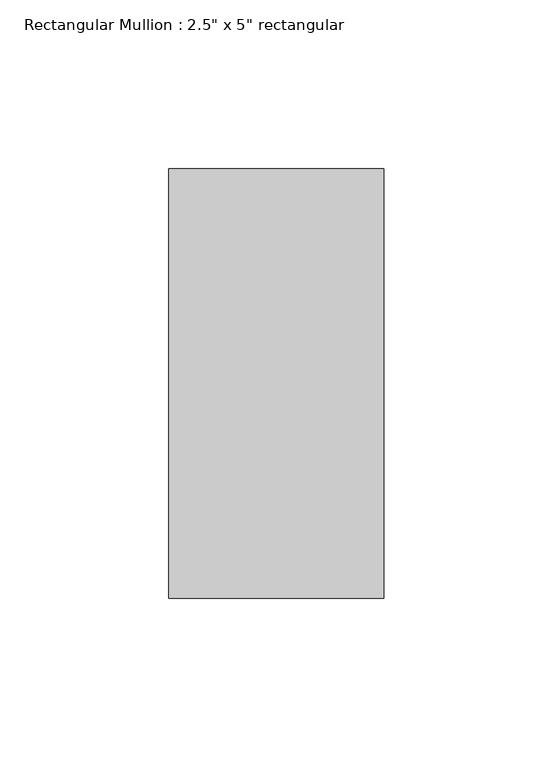
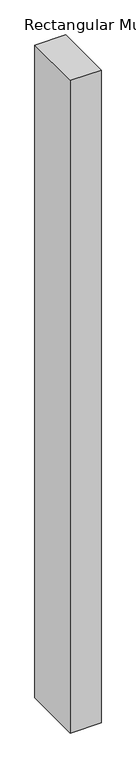
"""IFC4 building model written with IfcOpenShell, lengths in millimetres: member geometry."""

from ifc_helpers import new_model, si_unit, frame, origin, place, context, project, spatial, polyline, outline, extrude, source, transform, mapped, element, save


def member_347b2a6f(model_context):
    return source(origin(), model_context, "Body", "SweptSolid", [
        extrude(outline(polyline([(31.75, 63.5), (31.75, -63.5), (-31.75, -63.5), (-31.75, 63.5), (31.75, 63.5)])), frame((0.0, 0.0, -1428.2525568), z_axis=(0.0, 0.0, 1.0), x_axis=(1.0, 0.0, 0.0)), (0.0, 0.0, 1.0), 1428.2525568),
    ])


if __name__ == "__main__":
    model = new_model("IFC4")
    model_context = context("Model", 3, world=origin())
    ifc_project = project(units=[si_unit("LENGTHUNIT", "METRE", prefix="MILLI")], contexts=[model_context])
    site = spatial("IfcSite", under=ifc_project)
    building = spatial("IfcBuilding", under=site)
    placement = place(None, origin())
    member_shape = member_347b2a6f(model_context)
    element("IfcMember", 1, ObjectType="Rectangular Mullion : 2.5\" x 5\" rectangular", at=placement, inside=building, context=model_context, shape_type="MappedRepresentation", body=[
        mapped(member_shape, transform((0.0, 0.0, 0.0), x_axis=(1.0, 0.0, 0.0), y_axis=(0.0, 1.0, 0.0), z_axis=(0.0, 0.0, 1.0))),
    ])
    save(model, "model.ifc")

# Revit data of these elements
# Type "Rectangular Mullion : 2.5\" x 5\" rectangular"
#   built-in parameter 1007304 = 0.416667 (stored number, unit not read)
#   built-in parameter 1007301 = 0.104167 (stored number, unit not read)
#   built-in parameter 1007300 = 0.104167 (stored number, unit not read)
# Element 1 (IfcMember, "Rectangular Mullion : 2.5\" x 5\" rectangular")
#   Materials on its faces: "Aluminum"
# Materials
#   "Aluminum": class "Metal", colour RGB 247 247 247, transparency 0, Description = "Aluminum 6061", Cost = 0
